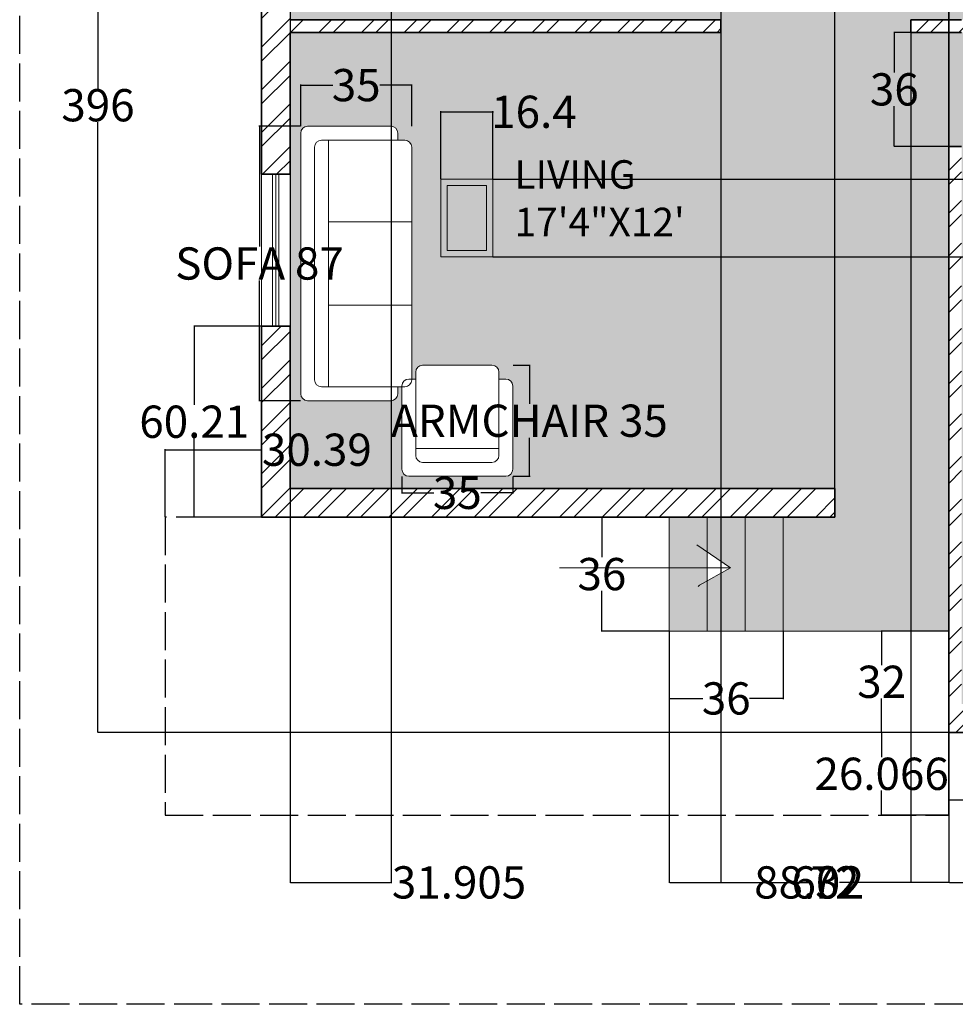
# Model space of a CAD drawing. Units: inches. Extents: x 1410 to 1959, y 5441 to 5968.
# Tile 1 of 5: x 1410 to 1705, y 5441 to 5751. Entities that reach past the tile are written whole.
import ezdxf

# ---------------------------------------------------------------- set-up
doc = ezdxf.new("R2010")
doc.units = ezdxf.units.IN
doc.linetypes.add('ACAD_ISO02W100', pattern=[15, 12, -3])
doc.layers.get('Defpoints').update_dxf_attribs({"linetype": 'ACAD_ISO02W100'})
for name, color, linetype, lineweight in [('00 FURNITURE', 15, 'Continuous', 15), ('A-ANNO-DIMS', 2, 'Continuous', 18), ('A-ANNO-SYMB', 7, 'Continuous', 18), ('A-AREA-IDEN', 7, 'Continuous', 18), ('A-FLOR-STRS', 7, 'Continuous', 18), ('A-WALL', 7, 'Continuous', 35), ('A-WALL-PATT', 8, 'Continuous', 13), ('WINDOW', 160, 'Continuous', 13)]:
    doc.layers.add(name, color=color, linetype=linetype, lineweight=lineweight)
for name, color, linetype, lineweight, true_color in [('A-FLOR-PATT', 9, 'Continuous', 9, 0xafd9aa), ('A-FLOR-STRS-PATT', 254, 'Continuous', 9, 0xddb3d4), ('A-FURN-PATT', 252, 'Continuous', 9, 0x939598)]:
    doc.layers.add(name, color=color, linetype=linetype, lineweight=lineweight, true_color=true_color)
doc.styles.get("Standard").update_dxf_attribs({"font": 'arial.ttf'})
doc.dimstyles.get("Standard").update_dxf_attribs({"dimtxt": 10.18, "dimasz": 0.18, "dimexe": 0.18, "dimexo": 0.0625, "dimgap": 0.09, "dimtad": 0, "dimtih": 1, "dimtoh": 1, "dimdec": 0, "dimzin": 0, "dimdsep": 46, "dimlunit": 3, "dimtxsty": 'Standard', "dimcen": 0.09, "dimadec": 0, "dimazin": 0, "dimtfac": 1, "dimtdec": 0, "dimtofl": 0, "dimtmove": 0, "dimatfit": 3, "dimfxl": 1, "dimtolj": 1, "dimtzin": 0, "dimarcsym": 0})

# ---------------------------------------------------------------- blocks, each defined once
blk = doc.blocks.new('sofa 6')
for p, q in [((-1044.4, 890), (1044.4, 890)), ((-1100, 166.9), (-1100, 834.3)), ((1100, 834.3), (1100, 166.9)), ((-988.8, 55.6), (-988.8, 723.1)), ((-933.1, 778.7), (933.1, 778.7)), ((988.8, 723.1), (988.8, 55.6)), ((-988.8, 667.5), (988.8, 667.5)), ((-333.8, 667.5), (-333.8, 0)), ((333.7, 667.5), (333.7, 0)), ((-988.8, 111.2), (-1044.4, 111.2)), ((1044.4, 111.2), (988.8, 111.2)), ((933.1, 0), (-933.1, 0))]:
    blk.add_line(p, q)
for centre, start, end in [((-1044.4, 834.3), 90, 180), ((1044.4, 834.3), 0, 90), ((-933.1, 723.1), 90, 180), ((933.1, 723.1), 0, 90), ((-1044.4, 166.9), 180, 270), ((1044.4, 166.9), 270, 0), ((-933.1, 55.6), 180, 270), ((933.1, 55.6), 270, 0)]:
    blk.add_arc(centre, 55.6, start, end)
blk = doc.blocks.new('CHAIR')
at = {"layer": '00 FURNITURE'}
for p, q in [((1776.1, 2600.27), (1776.1, 2626.55)), ((1778.29, 2628.74), (1800.19, 2628.74)), ((1802.38, 2626.55), (1802.38, 2600.27)), ((1773.91, 2624.36), (1776.1, 2624.36)), ((1802.38, 2624.36), (1804.57, 2624.36)), ((1771.72, 2595.89), (1771.72, 2622.17)), ((1806.76, 2622.17), (1806.76, 2595.89)), ((1802.38, 2602.46), (1776.1, 2602.46)), ((1800.19, 2598.08), (1778.29, 2598.08)), ((1804.57, 2593.7), (1773.91, 2593.7))]:
    blk.add_line(p, q, dxfattribs=at)
for centre, start, end in [((1778.29, 2626.55), 90, 180), ((1800.19, 2626.55), 0, 90), ((1773.91, 2622.17), 90, 180), ((1804.57, 2622.17), 0, 90), ((1778.29, 2600.27), 180, 270), ((1800.19, 2600.27), 270, 0), ((1773.91, 2595.89), 180, 270), ((1804.57, 2595.89), 270, 0)]:
    blk.add_arc(centre, 2.19, start, end, dxfattribs=at)
blk = doc.blocks.new('WIN-48IN')
for p, q in [((48, 9), (0, 9)), ((0, 5.5), (48, 5.5)), ((0, 4.5), (48, 4.5)), ((0, 3.5), (48, 3.5)), ((0, 0), (48, 0))]:
    blk.add_line(p, q)
blk = doc.blocks.new('*D16')
at = {"layer": 'A-ANNO-DIMS', "color": 0, "lineweight": -2, "transparency": 16777216}
for p, q in [((1498.38, 5717.72), (1485.27, 5717.72)), ((1485.45, 5717.54), (1485.45, 5679.77)), ((1485.45, 5631.29), (1485.45, 5669.06)), ((1498.38, 5631.11), (1485.27, 5631.11))]:
    blk.add_line(p, q, dxfattribs=at)
at = {"layer": 'A-ANNO-DIMS', "color": 0, "transparency": 16777216}
for points in [[(1485.42, 5717.54), (1485.48, 5717.54), (1485.45, 5717.72)], [(1485.42, 5631.29), (1485.48, 5631.29), (1485.45, 5631.11)]]:
    blk.add_solid(points, dxfattribs=at)
at = {"layer": 'Defpoints', "color": 0, "transparency": 16777216}
for p in [(1498.45, 5717.72), (1485.45, 5631.11), (1498.45, 5631.11)]:
    blk.add_point(p, dxfattribs=at)
at = {"layer": 'A-ANNO-DIMS', "color": 0, "transparency": 16777216, "insert": (1485.45, 5674.41), "char_height": 10.18, "attachment_point": 5}
blk.add_mtext('\\A1;SOFA 87', dxfattribs=at)
blk = doc.blocks.new('*D17')
at = {"layer": 'A-ANNO-DIMS', "color": 0, "lineweight": -2, "transparency": 16777216}
for p, q in [((1498.45, 5717.78), (1498.45, 5730.89)), ((1498.63, 5730.71), (1508.55, 5730.71)), ((1533.3, 5730.71), (1523.38, 5730.71)), ((1533.48, 5717.78), (1533.48, 5730.89))]:
    blk.add_line(p, q, dxfattribs=at)
at = {"layer": 'A-ANNO-DIMS', "color": 0, "transparency": 16777216}
for points in [[(1498.63, 5730.74), (1498.63, 5730.68), (1498.45, 5730.71)], [(1533.3, 5730.74), (1533.3, 5730.68), (1533.48, 5730.71)]]:
    blk.add_solid(points, dxfattribs=at)
at = {"layer": 'Defpoints', "color": 0, "transparency": 16777216}
for p in [(1498.45, 5730.71), (1498.45, 5717.72), (1533.48, 5717.72)]:
    blk.add_point(p, dxfattribs=at)
at = {"layer": 'A-ANNO-DIMS', "color": 0, "transparency": 16777216, "insert": (1515.97, 5730.71), "char_height": 10.18, "attachment_point": 5}
blk.add_mtext('\\A1;35', dxfattribs=at)
blk = doc.blocks.new('*D18')
at = {"layer": 'A-ANNO-DIMS', "color": 0, "lineweight": -2, "transparency": 16777216}
for p, q in [((1565.47, 5642.3), (1570.84, 5642.3)), ((1570.66, 5642.12), (1570.66, 5630.14)), ((1570.66, 5607.44), (1570.66, 5619.42)), ((1565.47, 5607.26), (1570.84, 5607.26))]:
    blk.add_line(p, q, dxfattribs=at)
at = {"layer": 'A-ANNO-DIMS', "color": 0, "transparency": 16777216}
for points in [[(1570.63, 5642.12), (1570.69, 5642.12), (1570.66, 5642.3)], [(1570.63, 5607.44), (1570.69, 5607.44), (1570.66, 5607.26)]]:
    blk.add_solid(points, dxfattribs=at)
at = {"layer": 'Defpoints', "color": 0, "transparency": 16777216}
for p in [(1565.4, 5642.3), (1570.66, 5642.3), (1565.4, 5607.26)]:
    blk.add_point(p, dxfattribs=at)
at = {"layer": 'A-ANNO-DIMS', "color": 0, "transparency": 16777216, "insert": (1570.66, 5624.78), "char_height": 10.18, "attachment_point": 5}
blk.add_mtext('\\A1;ARMCHAIR 35', dxfattribs=at)
blk = doc.blocks.new('*D19')
at = {"layer": 'A-ANNO-DIMS', "color": 0, "lineweight": -2, "transparency": 16777216}
for p, q in [((1530.37, 5607.2), (1530.37, 5601.83)), ((1565.4, 5607.2), (1565.4, 5601.83)), ((1530.55, 5602.01), (1540.47, 5602.01)), ((1565.22, 5602.01), (1555.3, 5602.01))]:
    blk.add_line(p, q, dxfattribs=at)
at = {"layer": 'A-ANNO-DIMS', "color": 0, "transparency": 16777216}
for points in [[(1530.55, 5602.04), (1530.55, 5601.98), (1530.37, 5602.01)], [(1565.22, 5602.04), (1565.22, 5601.98), (1565.4, 5602.01)]]:
    blk.add_solid(points, dxfattribs=at)
at = {"layer": 'Defpoints', "color": 0, "transparency": 16777216}
for p in [(1530.37, 5607.26), (1565.4, 5607.26), (1565.4, 5602.01)]:
    blk.add_point(p, dxfattribs=at)
at = {"layer": 'A-ANNO-DIMS', "color": 0, "transparency": 16777216, "insert": (1547.89, 5602.01), "char_height": 10.18, "attachment_point": 5}
blk.add_mtext('\\A1;35', dxfattribs=at)
blk = doc.blocks.new('*D25')
at = {"layer": 'A-ANNO-DIMS', "color": 0, "lineweight": -2, "transparency": 16777216}
for p, q in [((1486.03, 5922.37), (1434.27, 5922.37)), ((1434.45, 5922.19), (1434.45, 5729.66)), ((1434.45, 5526.55), (1434.45, 5719.07)), ((1703.03, 5526.37), (1434.27, 5526.37))]:
    blk.add_line(p, q, dxfattribs=at)
at = {"layer": 'A-ANNO-DIMS', "color": 0, "transparency": 16777216}
for points in [[(1434.42, 5922.19), (1434.48, 5922.19), (1434.45, 5922.37)], [(1434.42, 5526.55), (1434.48, 5526.55), (1434.45, 5526.37)]]:
    blk.add_solid(points, dxfattribs=at)
at = {"layer": 'Defpoints', "color": 0, "transparency": 16777216}
for p in [(1434.45, 5922.37), (1486.09, 5922.37), (1703.09, 5526.37)]:
    blk.add_point(p, dxfattribs=at)
at = {"layer": 'A-ANNO-DIMS', "color": 0, "transparency": 16777216, "insert": (1434.45, 5724.37), "char_height": 10.18, "attachment_point": 5}
blk.add_mtext('\\A1;396', dxfattribs=at)
blk = doc.blocks.new('*D26')
at = {"layer": 'A-ANNO-DIMS', "color": 0, "lineweight": -2, "transparency": 16777216}
for p, q in [((1703.09, 5526.3), (1703.09, 5478.87)), ((1858.09, 5526.3), (1858.09, 5478.87)), ((1703.27, 5479.05), (1769.7, 5479.05)), ((1857.91, 5479.05), (1791.49, 5479.05))]:
    blk.add_line(p, q, dxfattribs=at)
at = {"layer": 'A-ANNO-DIMS', "color": 0, "transparency": 16777216}
for points in [[(1703.27, 5479.08), (1703.27, 5479.02), (1703.09, 5479.05)], [(1857.91, 5479.08), (1857.91, 5479.02), (1858.09, 5479.05)]]:
    blk.add_solid(points, dxfattribs=at)
at = {"layer": 'Defpoints', "color": 0, "transparency": 16777216}
for p in [(1703.09, 5526.37), (1858.09, 5526.37), (1858.09, 5479.05)]:
    blk.add_point(p, dxfattribs=at)
at = {"layer": 'A-ANNO-DIMS', "color": 0, "transparency": 16777216, "insert": (1780.59, 5479.05), "char_height": 10.18, "attachment_point": 5}
blk.add_mtext('\\A1;155', dxfattribs=at)
blk = doc.blocks.new('*D27')
at = {"layer": 'A-ANNO-DIMS', "color": 0, "lineweight": -2, "transparency": 16777216}
for p, q in [((1495.09, 5913.3), (1495.09, 5478.87)), ((1527, 5913.3), (1527, 5478.87)), ((1495.27, 5479.05), (1526.82, 5479.05)), ((1527, 5479.05), (1527.18, 5479.05))]:
    blk.add_line(p, q, dxfattribs=at)
at = {"layer": 'A-ANNO-DIMS', "color": 0, "transparency": 16777216}
for points in [[(1495.27, 5479.08), (1495.27, 5479.02), (1495.09, 5479.05)], [(1526.82, 5479.08), (1526.82, 5479.02), (1527, 5479.05)]]:
    blk.add_solid(points, dxfattribs=at)
at = {"layer": 'Defpoints', "color": 0, "transparency": 16777216}
for p in [(1495.09, 5913.37), (1527, 5913.37), (1527, 5479.05)]:
    blk.add_point(p, dxfattribs=at)
at = {"layer": 'A-ANNO-DIMS', "color": 0, "transparency": 16777216, "insert": (1548.43, 5479.05), "char_height": 10.18, "attachment_point": 5}
blk.add_mtext('\\A1;31.905', dxfattribs=at)
blk = doc.blocks.new('*D30')
at = {"layer": 'A-ANNO-DIMS', "color": 0, "lineweight": -2, "transparency": 16777216}
for p, q in [((1486.04, 5654.58), (1464.67, 5654.58)), ((1464.85, 5654.4), (1464.85, 5629.76)), ((1464.84, 5594.55), (1464.85, 5619.19)), ((1486.03, 5594.37), (1464.66, 5594.37))]:
    blk.add_line(p, q, dxfattribs=at)
at = {"layer": 'A-ANNO-DIMS', "color": 0, "transparency": 16777216}
for points in [[(1464.82, 5654.4), (1464.88, 5654.4), (1464.85, 5654.58)], [(1464.81, 5594.55), (1464.87, 5594.55), (1464.84, 5594.37)]]:
    blk.add_solid(points, dxfattribs=at)
at = {"layer": 'Defpoints', "color": 0, "transparency": 16777216}
for p in [(1464.85, 5654.58), (1486.1, 5654.58), (1486.09, 5594.37)]:
    blk.add_point(p, dxfattribs=at)
at = {"layer": 'A-ANNO-DIMS', "color": 0, "transparency": 16777216, "insert": (1464.85, 5624.47), "char_height": 10.18, "attachment_point": 5}
blk.add_mtext('\\A1;60.21', dxfattribs=at)
blk = doc.blocks.new('*D31')
at = {"layer": 'A-ANNO-DIMS', "color": 0, "lineweight": -2, "transparency": 16777216}
for p, q in [((1703.09, 5526.3), (1703.09, 5504.94)), ((1754.54, 5526.3), (1754.54, 5504.94)), ((1703.27, 5505.12), (1711.51, 5505.12)), ((1754.36, 5505.12), (1746.12, 5505.12))]:
    blk.add_line(p, q, dxfattribs=at)
at = {"layer": 'A-ANNO-DIMS', "color": 0, "transparency": 16777216}
for points in [[(1703.27, 5505.15), (1703.27, 5505.09), (1703.09, 5505.12)], [(1754.36, 5505.15), (1754.36, 5505.09), (1754.54, 5505.12)]]:
    blk.add_solid(points, dxfattribs=at)
at = {"layer": 'Defpoints', "color": 0, "transparency": 16777216}
for p in [(1703.09, 5526.37), (1754.54, 5526.37), (1703.09, 5505.12)]:
    blk.add_point(p, dxfattribs=at)
at = {"layer": 'A-ANNO-DIMS', "color": 0, "transparency": 16777216, "insert": (1728.82, 5505.12), "char_height": 10.18, "attachment_point": 5}
blk.add_mtext('\\A1;51.45', dxfattribs=at)
blk = doc.blocks.new('*D34')
at = {"layer": 'A-ANNO-DIMS', "color": 0, "lineweight": -2, "transparency": 16777216}
for p, q in [((1631.09, 5787.3), (1631.09, 5478.87)), ((1703.09, 5787.3), (1703.09, 5478.87)), ((1631.27, 5479.05), (1659.81, 5479.05)), ((1702.91, 5479.05), (1674.38, 5479.05))]:
    blk.add_line(p, q, dxfattribs=at)
at = {"layer": 'A-ANNO-DIMS', "color": 0, "transparency": 16777216}
for points in [[(1631.27, 5479.08), (1631.27, 5479.02), (1631.09, 5479.05)], [(1702.91, 5479.08), (1702.91, 5479.02), (1703.09, 5479.05)]]:
    blk.add_solid(points, dxfattribs=at)
at = {"layer": 'Defpoints', "color": 0, "transparency": 16777216}
for p in [(1631.09, 5787.37), (1703.09, 5787.37), (1703.09, 5479.05)]:
    blk.add_point(p, dxfattribs=at)
at = {"layer": 'A-ANNO-DIMS', "color": 0, "transparency": 16777216, "insert": (1667.09, 5479.05), "char_height": 10.18, "attachment_point": 5}
blk.add_mtext('\\A1;72', dxfattribs=at)
blk = doc.blocks.new('*D36')
at = {"layer": 'A-ANNO-DIMS', "color": 0, "lineweight": -2, "transparency": 16777216}
for p, q in [((1631.09, 5747.3), (1631.09, 5478.87)), ((1691.09, 5747.3), (1691.09, 5478.87)), ((1631.27, 5479.05), (1653.7, 5479.05)), ((1690.91, 5479.05), (1668.49, 5479.05))]:
    blk.add_line(p, q, dxfattribs=at)
at = {"layer": 'A-ANNO-DIMS', "color": 0, "transparency": 16777216}
for points in [[(1631.27, 5479.08), (1631.27, 5479.02), (1631.09, 5479.05)], [(1690.91, 5479.08), (1690.91, 5479.02), (1691.09, 5479.05)]]:
    blk.add_solid(points, dxfattribs=at)
at = {"layer": 'Defpoints', "color": 0, "transparency": 16777216}
for p in [(1631.09, 5747.37), (1691.09, 5747.37), (1691.09, 5479.05)]:
    blk.add_point(p, dxfattribs=at)
at = {"layer": 'A-ANNO-DIMS', "color": 0, "transparency": 16777216, "insert": (1661.09, 5479.05), "char_height": 10.18, "attachment_point": 5}
blk.add_mtext('\\A1;60', dxfattribs=at)
blk = doc.blocks.new('*D37')
at = {"layer": 'A-ANNO-DIMS', "color": 0, "lineweight": -2, "transparency": 16777216}
for p, q in [((1667.09, 5594.43), (1667.09, 5943.8)), ((1667.27, 5943.62), (1677.72, 5943.62)), ((1702.91, 5943.62), (1692.47, 5943.62)), ((1703.09, 5558.43), (1703.09, 5943.8))]:
    blk.add_line(p, q, dxfattribs=at)
at = {"layer": 'A-ANNO-DIMS', "color": 0, "transparency": 16777216}
for points in [[(1667.27, 5943.65), (1667.27, 5943.59), (1667.09, 5943.62)], [(1702.91, 5943.65), (1702.91, 5943.59), (1703.09, 5943.62)]]:
    blk.add_solid(points, dxfattribs=at)
at = {"layer": 'Defpoints', "color": 0, "transparency": 16777216}
for p in [(1703.09, 5943.62), (1667.09, 5594.37), (1703.09, 5558.37)]:
    blk.add_point(p, dxfattribs=at)
at = {"layer": 'A-ANNO-DIMS', "color": 0, "transparency": 16777216, "insert": (1685.09, 5943.62), "char_height": 10.18, "attachment_point": 5}
blk.add_mtext('\\A1;36', dxfattribs=at)
blk = doc.blocks.new('*D38')
at = {"layer": 'A-ANNO-DIMS', "color": 0, "lineweight": -2, "transparency": 16777216}
for p, q in [((1614.72, 5594.37), (1593.35, 5594.37)), ((1593.53, 5594.19), (1593.53, 5581.66)), ((1593.53, 5558.55), (1593.53, 5571.07)), ((1614.72, 5558.37), (1593.35, 5558.37))]:
    blk.add_line(p, q, dxfattribs=at)
at = {"layer": 'A-ANNO-DIMS', "color": 0, "transparency": 16777216}
for points in [[(1593.5, 5594.19), (1593.56, 5594.19), (1593.53, 5594.37)], [(1593.5, 5558.55), (1593.56, 5558.55), (1593.53, 5558.37)]]:
    blk.add_solid(points, dxfattribs=at)
at = {"layer": 'Defpoints', "color": 0, "transparency": 16777216}
for p in [(1593.53, 5594.37), (1614.78, 5594.37), (1614.78, 5558.37)]:
    blk.add_point(p, dxfattribs=at)
at = {"layer": 'A-ANNO-DIMS', "color": 0, "transparency": 16777216, "insert": (1593.53, 5576.37), "char_height": 10.18, "attachment_point": 5}
blk.add_mtext('\\A1;36', dxfattribs=at)
blk = doc.blocks.new('*D39')
at = {"layer": 'A-ANNO-DIMS', "color": 0, "lineweight": -2, "transparency": 16777216}
for p, q in [((1614.78, 5558.3), (1614.78, 5478.87)), ((1703.09, 5558.3), (1703.09, 5478.87)), ((1614.96, 5479.05), (1641.72, 5479.05)), ((1702.91, 5479.05), (1676.16, 5479.05))]:
    blk.add_line(p, q, dxfattribs=at)
at = {"layer": 'A-ANNO-DIMS', "color": 0, "transparency": 16777216}
for points in [[(1614.96, 5479.08), (1614.96, 5479.02), (1614.78, 5479.05)], [(1702.91, 5479.08), (1702.91, 5479.02), (1703.09, 5479.05)]]:
    blk.add_solid(points, dxfattribs=at)
at = {"layer": 'Defpoints', "color": 0, "transparency": 16777216}
for p in [(1614.78, 5558.37), (1703.09, 5558.37), (1703.09, 5479.05)]:
    blk.add_point(p, dxfattribs=at)
at = {"layer": 'A-ANNO-DIMS', "color": 0, "transparency": 16777216, "insert": (1658.94, 5479.05), "char_height": 10.18, "attachment_point": 5}
blk.add_mtext('\\A1;88.32', dxfattribs=at)
blk = doc.blocks.new('*D40')
at = {"layer": 'A-ANNO-DIMS', "color": 0, "lineweight": -2, "transparency": 16777216}
for p, q in [((1703.03, 5558.37), (1681.66, 5558.37)), ((1681.84, 5558.19), (1681.84, 5547.66)), ((1681.84, 5526.55), (1681.84, 5537.07)), ((1703.03, 5526.37), (1681.66, 5526.37))]:
    blk.add_line(p, q, dxfattribs=at)
at = {"layer": 'A-ANNO-DIMS', "color": 0, "transparency": 16777216}
for points in [[(1681.81, 5558.19), (1681.87, 5558.19), (1681.84, 5558.37)], [(1681.81, 5526.55), (1681.87, 5526.55), (1681.84, 5526.37)]]:
    blk.add_solid(points, dxfattribs=at)
at = {"layer": 'Defpoints', "color": 0, "transparency": 16777216}
for p in [(1681.84, 5558.37), (1703.09, 5558.37), (1703.09, 5526.37)]:
    blk.add_point(p, dxfattribs=at)
at = {"layer": 'A-ANNO-DIMS', "color": 0, "transparency": 16777216, "insert": (1681.84, 5542.37), "char_height": 10.18, "attachment_point": 5}
blk.add_mtext('\\A1;32', dxfattribs=at)
blk = doc.blocks.new('*D47')
at = {"layer": 'A-ANNO-DIMS', "color": 0, "lineweight": -2, "transparency": 16777216}
for p, q in [((1707.03, 5747.37), (1685.66, 5747.37)), ((1685.84, 5747.19), (1685.84, 5734.66)), ((1685.84, 5711.55), (1685.84, 5724.07)), ((1707.03, 5711.37), (1685.66, 5711.37))]:
    blk.add_line(p, q, dxfattribs=at)
at = {"layer": 'A-ANNO-DIMS', "color": 0, "transparency": 16777216}
for points in [[(1685.81, 5747.19), (1685.87, 5747.19), (1685.84, 5747.37)], [(1685.81, 5711.55), (1685.87, 5711.55), (1685.84, 5711.37)]]:
    blk.add_solid(points, dxfattribs=at)
at = {"layer": 'Defpoints', "color": 0, "transparency": 16777216}
for p in [(1685.84, 5747.37), (1707.09, 5747.37), (1707.09, 5711.37)]:
    blk.add_point(p, dxfattribs=at)
at = {"layer": 'A-ANNO-DIMS', "color": 0, "transparency": 16777216, "insert": (1685.84, 5729.37), "char_height": 10.18, "attachment_point": 5}
blk.add_mtext('\\A1;36', dxfattribs=at)
blk = doc.blocks.new('*D53')
at = {"layer": 'A-ANNO-DIMS', "color": 0, "lineweight": -2, "transparency": 16777216}
for p, q in [((1455.7, 5594.43), (1455.7, 5615.8)), ((1455.88, 5615.62), (1485.92, 5615.62)), ((1486.09, 5594.43), (1486.1, 5615.8)), ((1486.1, 5615.62), (1486.28, 5615.62))]:
    blk.add_line(p, q, dxfattribs=at)
at = {"layer": 'A-ANNO-DIMS', "color": 0, "transparency": 16777216}
for points in [[(1455.88, 5615.65), (1455.88, 5615.59), (1455.7, 5615.62)], [(1485.92, 5615.65), (1485.92, 5615.59), (1486.1, 5615.62)]]:
    blk.add_solid(points, dxfattribs=at)
at = {"layer": 'Defpoints', "color": 0, "transparency": 16777216}
for p in [(1486.1, 5615.62), (1455.7, 5594.37), (1486.09, 5594.37)]:
    blk.add_point(p, dxfattribs=at)
at = {"layer": 'A-ANNO-DIMS', "color": 0, "transparency": 16777216, "insert": (1503.55, 5615.62), "char_height": 10.18, "attachment_point": 5}
blk.add_mtext('\\A1;30.39', dxfattribs=at)
blk = doc.blocks.new('*D54')
at = {"layer": 'A-ANNO-DIMS', "color": 0, "lineweight": -2, "transparency": 16777216}
for p, q in [((1703.03, 5526.37), (1681.66, 5526.37)), ((1681.84, 5526.19), (1681.84, 5518.62)), ((1681.84, 5500.48), (1681.84, 5508.05)), ((1703.03, 5500.3), (1681.66, 5500.3))]:
    blk.add_line(p, q, dxfattribs=at)
at = {"layer": 'A-ANNO-DIMS', "color": 0, "transparency": 16777216}
for points in [[(1681.81, 5526.19), (1681.87, 5526.19), (1681.84, 5526.37)], [(1681.81, 5500.48), (1681.87, 5500.48), (1681.84, 5500.3)]]:
    blk.add_solid(points, dxfattribs=at)
at = {"layer": 'Defpoints', "color": 0, "transparency": 16777216}
for p in [(1681.84, 5526.37), (1703.09, 5526.37), (1703.09, 5500.3)]:
    blk.add_point(p, dxfattribs=at)
at = {"layer": 'A-ANNO-DIMS', "color": 0, "transparency": 16777216, "insert": (1681.84, 5513.33), "char_height": 10.18, "attachment_point": 5}
blk.add_mtext('\\A1;26.066', dxfattribs=at)
blk = doc.blocks.new('*D55')
at = {"layer": 'A-ANNO-DIMS', "color": 0, "lineweight": -2, "transparency": 16777216}
for p, q in [((1614.78, 5558.3), (1614.78, 5536.94)), ((1650.78, 5558.3), (1650.78, 5536.94)), ((1614.96, 5537.12), (1625.4, 5537.12)), ((1650.6, 5537.12), (1640.15, 5537.12))]:
    blk.add_line(p, q, dxfattribs=at)
at = {"layer": 'A-ANNO-DIMS', "color": 0, "transparency": 16777216}
for points in [[(1614.96, 5537.15), (1614.96, 5537.09), (1614.78, 5537.12)], [(1650.6, 5537.15), (1650.6, 5537.09), (1650.78, 5537.12)]]:
    blk.add_solid(points, dxfattribs=at)
at = {"layer": 'Defpoints', "color": 0, "transparency": 16777216}
for p in [(1614.78, 5558.37), (1650.78, 5558.37), (1614.78, 5537.12)]:
    blk.add_point(p, dxfattribs=at)
at = {"layer": 'A-ANNO-DIMS', "color": 0, "transparency": 16777216, "insert": (1632.78, 5537.12), "char_height": 10.18, "attachment_point": 5}
blk.add_mtext('\\A1;36', dxfattribs=at)
blk = doc.blocks.new('*D59')
at = {"layer": 'A-ANNO-DIMS', "color": 0, "lineweight": -2, "transparency": 16777216}
for p, q in [((1559.15, 5701.04), (1879.55, 5701.04)), ((1879.37, 5700.86), (1879.37, 5694.04)), ((1879.37, 5676.64), (1879.37, 5683.46)), ((1559.15, 5676.46), (1879.55, 5676.46))]:
    blk.add_line(p, q, dxfattribs=at)
at = {"layer": 'A-ANNO-DIMS', "color": 0, "transparency": 16777216}
for points in [[(1879.34, 5700.86), (1879.4, 5700.86), (1879.37, 5701.04)], [(1879.34, 5676.64), (1879.4, 5676.64), (1879.37, 5676.46)]]:
    blk.add_solid(points, dxfattribs=at)
at = {"layer": 'Defpoints', "color": 0, "transparency": 16777216}
for p in [(1559.09, 5701.04), (1559.09, 5676.46), (1879.37, 5676.46)]:
    blk.add_point(p, dxfattribs=at)
at = {"layer": 'A-ANNO-DIMS', "color": 0, "transparency": 16777216, "insert": (1879.37, 5688.75), "char_height": 10.18, "attachment_point": 5}
blk.add_mtext('\\A1;24.58', dxfattribs=at)
blk = doc.blocks.new('*D60')
at = {"layer": 'A-ANNO-DIMS', "color": 0, "lineweight": -2, "transparency": 16777216}
for p, q in [((1542.69, 5701.1), (1542.69, 5722.47)), ((1542.87, 5722.29), (1558.91, 5722.29)), ((1559.09, 5701.1), (1559.09, 5722.47)), ((1559.09, 5722.29), (1559.27, 5722.29))]:
    blk.add_line(p, q, dxfattribs=at)
at = {"layer": 'A-ANNO-DIMS', "color": 0, "transparency": 16777216}
for points in [[(1542.87, 5722.32), (1542.87, 5722.26), (1542.69, 5722.29)], [(1558.91, 5722.32), (1558.91, 5722.26), (1559.09, 5722.29)]]:
    blk.add_solid(points, dxfattribs=at)
at = {"layer": 'Defpoints', "color": 0, "transparency": 16777216}
for p in [(1559.09, 5722.29), (1542.69, 5701.04), (1559.09, 5701.04)]:
    blk.add_point(p, dxfattribs=at)
at = {"layer": 'A-ANNO-DIMS', "color": 0, "transparency": 16777216, "insert": (1572.08, 5722.29), "char_height": 10.18, "attachment_point": 5}
blk.add_mtext('\\A1;16.4', dxfattribs=at)

msp = doc.modelspace()

# ---------------------------------------------------------------- hatches: boundary and pattern name
at = {"layer": 'A-FLOR-PATT', "transparency": 33554534}
h = msp.add_hatch(color=256, dxfattribs=at)
h.dxf.hatch_style = 1
h.paths.add_polyline_path([(1849.0942, 5913.3659), (1817.1029, 5913.3659), (1769.1029, 5913.3659), (1769.1029, 5913.3659), (1707.0942, 5913.3659), (1707.0942, 5787.3659), (1703.0942, 5787.3659), (1703.0942, 5799.3659), (1631.0942, 5799.3659), (1631.0942, 5787.3659), (1627.0942, 5787.3659), (1627.0942, 5889.3659), (1519.0989, 5889.3659), (1519.0989, 5816.4745), (1495.0981, 5816.4745), (1495.0981, 5809.856), (1495.0942, 5751.3659), (1631.0942, 5751.3659), (1631.0942, 5747.3659), (1495.0942, 5747.3659), (1495.0942, 5702.5811), (1495.0984, 5654.5768), (1495.0942, 5603.3659), (1667.0942, 5603.3659), (1667.0942, 5594.3659), (1650.778, 5594.3659), (1650.778, 5558.3659), (1703.0942, 5558.3659), (1703.0942, 5594.3659), (1703.0942, 5711.3659), (1707.0942, 5711.3659), (1707.0942, 5535.3659), (1754.5413, 5535.3659), (1802.541, 5535.3658), (1802.5413, 5535.3658), (1802.5413, 5535.3659), (1849.0942, 5535.3659), (1849.0942, 5651.3659), (1743.0942, 5651.3659), (1743.0942, 5655.3659), (1849.0942, 5655.3659), (1849.0942, 5665.4579), (1849.0942, 5689.4579), (1849.0942, 5699.3659), (1801.0942, 5699.3659), (1801.0942, 5685.3659), (1797.0942, 5685.3659), (1797.0942, 5699.3659), (1783.0942, 5699.3659), (1783.0942, 5703.3659), (1849.0942, 5703.3659), (1849.0942, 5716.9764), (1849.123, 5716.9764), (1849.123, 5740.9654), (1849.0942, 5740.9654), (1849.0942, 5747.3659), (1753.0942, 5747.3659), (1753.0942, 5699.3659), (1749.0942, 5699.3659), (1749.0942, 5747.3659), (1707.0942, 5747.3659), (1691.0942, 5747.3659), (1691.0942, 5751.3659), (1707.0942, 5751.3659), (1849.0942, 5751.3659)])
h.paths.add_polyline_path([(1533.4842, 5711.1518), (1533.4842, 5637.9201), (1534.7464, 5637.9201), (1534.7464, 5640.1099, -0.41421356), (1536.9363, 5642.2998), (1558.8347, 5642.2998, -0.41421356), (1561.0246, 5640.1099), (1561.0246, 5637.9201), (1563.2144, 5637.9201, -0.41421356), (1565.4042, 5635.7302), (1565.4042, 5609.4519, -0.41421356), (1563.2144, 5607.2621), (1532.5566, 5607.2621, -0.41421356), (1530.3668, 5609.4519), (1530.3668, 5635.4862), (1529.1045, 5635.4862), (1529.1045, 5633.2964, -0.41421356), (1526.9147, 5631.1065), (1500.6363, 5631.1065, -0.41421356), (1498.4465, 5633.2964), (1498.4465, 5715.5315, -0.41421356), (1500.6363, 5717.7213), (1526.9147, 5717.7213, -0.41421356), (1529.1045, 5715.5315), (1529.1045, 5713.3417), (1531.2944, 5713.3417, -0.41421356)], flags=16)
h.paths.add_polyline_path([(1771.0631, 5793.9619), (1771.0631, 5835.0118), (1771.0631, 5856.9619, -0.41421356), (1771.9631, 5857.8619), (1842.1181, 5857.8619, -0.41421356), (1843.0181, 5856.9619), (1843.0181, 5857.8619), (1846.6631, 5857.8619), (1846.6631, 5793.0619), (1843.0181, 5793.0619), (1828.4381, 5793.0619), (1771.9631, 5793.0619, -0.41421356)], flags=16)
h.paths.add_polyline_path([(1771.0631, 5805.9671, 0.25346465), (1781.0166, 5803.0153, 0.25379956), (1783.9781, 5793.0522)], flags=16)
h.paths.add_polyline_path([(1746.3058, 5612.0795), (1768.2559, 5612.0795), (1809.3058, 5612.0795, -0.41421356), (1810.2058, 5611.1795), (1810.2058, 5554.7045), (1810.2058, 5540.1245), (1810.2058, 5536.4795), (1745.4058, 5536.4795), (1745.4058, 5540.1245), (1746.3058, 5540.1245, -0.41421356), (1745.4058, 5541.0245), (1745.4058, 5611.1795, -0.41421356)], flags=16)
h.paths.add_polyline_path([(1819.5646, 5793.1537), (1819.5646, 5793.8054, 0.05271893), (1808.0815, 5849.0458, 0.29223153), (1819.5646, 5857.6981), (1828.4381, 5857.6981), (1828.4381, 5857.0464), (1828.4381, 5847.601, -0.06332793), (1838.1593, 5837.9401, -0.38046479), (1838.3062, 5835.5217, -0.02593615), (1834.5989, 5831.2824, -0.02509022), (1838.1593, 5827.1584, -0.38046478), (1838.3062, 5824.74, -0.05941785), (1829.2061, 5815.646, -0.11763956), (1828.4381, 5815.2914), (1828.4381, 5793.1537)], flags=0)
h.paths.add_polyline_path([(1819.5646, 5793.1537), (1819.5646, 5822.5662, -0.01603557), (1817.3363, 5825.2436, -0.4295765), (1817.4052, 5827.8865, -0.01537126), (1819.5646, 5830.4335), (1819.5646, 5833.3479, -0.01603557), (1817.3363, 5836.0254, -0.48413611), (1817.6682, 5838.8652, 0.00079305), (1817.0318, 5838.199, 0.26524804), (1817.0526, 5836.3926, 0.02736634), (1820.9176, 5831.8795, 0.02734261), (1817.0221, 5827.3996, 0.26229506), (1817.0526, 5825.6108, 0.06555279), (1827.0712, 5815.5721), (1827.0712, 5793.1537)], flags=0)
h.paths.add_polyline_path([(1830.4631, 5775.9619), (1830.4631, 5792.1619), (1846.6631, 5792.1619), (1846.6631, 5775.9619)], flags=16)
h.paths.add_polyline_path([(1831.3631, 5776.8619), (1831.3631, 5791.2619), (1845.7631, 5791.2619), (1845.7631, 5776.8619)], flags=0)
h.paths.add_polyline_path([(1836.6983, 5784.1006, -1), (1843.9547, 5784.1006, -1)], flags=0)
h.paths.add_polyline_path([(1819.2615, 5682.5311, -0.25820517), (1830.2865, 5687.0962, -0.1716359), (1835.799, 5683.9093), (1838.1615, 5683.9093), (1838.1615, 5688.0436, -0.41421356), (1839.1458, 5689.028), (1845.4458, 5689.028, -0.41421356), (1846.4302, 5688.0436), (1846.4302, 5671.8999, -0.41421356), (1845.4458, 5670.9155), (1839.1458, 5670.9155, -0.41421356), (1838.1615, 5671.8999), (1838.1615, 5676.0343), (1835.799, 5676.0343, -0.1716359), (1830.2865, 5672.8474, -0.25820517), (1819.2615, 5677.4124)], flags=16)
h.paths.add_polyline_path([(1820.8043, 5682.5681, -0.21038447), (1830.2865, 5685.5212, -0.1716359), (1835.799, 5682.3343), (1835.799, 5677.6093, -0.1716359), (1830.2865, 5674.4224, -0.21038447), (1820.8043, 5677.3755)], flags=0)
h.paths.add_polyline_path([(1842.0614, 5784.0231), (1841.8811, 5784.0231, -0.54460611), (1839.6163, 5782.7155), (1839.5262, 5782.5594, 0.54796211)], flags=0)
h.paths.add_polyline_path([(1840.3713, 5784.1781), (1840.3265, 5784.2556), (1840.2818, 5784.1781)], flags=0)
h.paths.add_polyline_path([(1830.4631, 5858.7619), (1830.4631, 5874.9619), (1846.6631, 5874.9619), (1846.6631, 5858.7619)], flags=16)
h.paths.add_polyline_path([(1831.3631, 5859.6619), (1831.3631, 5874.0619), (1845.7631, 5874.0619), (1845.7631, 5859.6619)], flags=0)
h.paths.add_polyline_path([(1755.6206, 5556.6903, -0.00089292), (1756.3396, 5557.4382), (1745.5695, 5557.4382), (1745.5695, 5554.7045), (1746.2212, 5554.7045), (1755.5673, 5554.7045, -0.38881883)], flags=0)
h.paths.add_polyline_path([(1810.114, 5563.578), (1810.114, 5554.7045), (1809.4622, 5554.7045), (1787.9762, 5554.7045, -0.11778508), (1787.6251, 5553.9338, -0.05941785), (1778.5249, 5544.8398, -0.37985907), (1776.1092, 5544.9833, -0.02509022), (1771.9852, 5548.5437, 0.03343123), (1776.8399, 5553.9365, 0.30845915), (1776.98, 5555.985, 0.04782679), (1769.9197, 5563.578), (1772.8341, 5563.578, -0.01537126), (1775.3811, 5565.7373, -0.4295765), (1778.024, 5565.8063, -0.01603557), (1780.7015, 5563.578)], flags=0)
h.paths.add_polyline_path([(1728.3058, 5552.6795), (1744.5058, 5552.6795), (1744.5058, 5536.4795), (1728.3058, 5536.4795)], flags=16)
h.paths.add_polyline_path([(1810.2058, 5599.1742, 0.25346465), (1800.2523, 5602.126, 0.25379956), (1797.2908, 5612.0892)], flags=16)
h.paths.add_polyline_path([(1843.9547, 5866.8231, -1), (1836.6983, 5866.8231, -1)], flags=0)
h.paths.add_polyline_path([(1729.2058, 5551.7795), (1743.6058, 5551.7795), (1743.6058, 5537.3795), (1729.2058, 5537.3795)], flags=0)
h.paths.add_polyline_path([(1839.4821, 5865.5155), (1840.237, 5866.8231), (1839.4821, 5868.1307, 0.25464572), (1838.77, 5866.8231, 0.25464572)], flags=0)
h.paths.add_polyline_path([(1842.0614, 5866.7456), (1840.3713, 5866.7456), (1839.5262, 5865.2819, 0.54796211)], flags=0)
h.paths.add_polyline_path([(1732.8163, 5542.8161, -1), (1740.0727, 5542.8161, -1)], flags=0)
h.paths.add_polyline_path([(1737.8296, 5543.5262), (1736.522, 5542.7713), (1736.522, 5541.2615, 0.39969799), (1738.001, 5542.8161, 0.11900365)], flags=0)
h.paths.add_polyline_path([(1738.1811, 5542.8161, -1), (1734.7079, 5542.8161, -1)], flags=0)
h.paths.add_polyline_path([(1736.4445, 5542.9056), (1736.367, 5542.9503), (1736.367, 5542.8608)], flags=0)
h.paths.add_polyline_path([(1811.1058, 5552.6795), (1827.3058, 5552.6795), (1827.3058, 5536.4795), (1811.1058, 5536.4795)], flags=16)
h.paths.add_polyline_path([(1812.0058, 5551.7795), (1826.4058, 5551.7795), (1826.4058, 5537.3795), (1812.0058, 5537.3795)], flags=0)
h.paths.add_polyline_path([(1815.5388, 5542.8161, -1), (1822.7952, 5542.8161, -1)], flags=0)
h.paths.add_polyline_path([(1820.5521, 5543.5262), (1819.2445, 5542.7713), (1819.2445, 5541.2615, 0.39969799), (1820.7235, 5542.8161, 0.11900365)], flags=0)
h.paths.add_polyline_path([(1820.9036, 5542.8161, -1), (1817.4304, 5542.8161, -1)], flags=0)
h.paths.add_polyline_path([(1819.167, 5542.9056), (1819.0895, 5542.9503), (1819.0895, 5542.8608)], flags=0)
h.paths.add_polyline_path([(1707.0264, 5710.8395), (1750.0905, 5710.8395), (1750.0905, 5723.2037), (1707.0264, 5723.2037)], flags=25)
h.paths.add_polyline_path([(1786.4108, 5658.162), (1818.7518, 5658.162), (1818.7518, 5680.5262), (1786.4108, 5680.5262)], flags=24)
h.paths.add_polyline_path([(1787.0609, 5715.7465), (1838.4906, 5715.7465), (1838.4906, 5738.1353), (1787.0609, 5738.1353)], flags=24)
h.paths.add_polyline_path([(1743.8116, 5616.0244), (1813.7243, 5616.0244), (1813.7243, 5649.6076), (1743.8116, 5649.6076)], flags=24)
h.paths.add_polyline_path([(1719.2569, 5867.7974), (1789.1696, 5867.7974), (1789.1696, 5901.3806), (1719.2569, 5901.3806)], flags=24)
h.paths.add_polyline_path([(1562.3198, 5677.907), (1619.4324, 5677.907), (1619.4324, 5711.4902), (1562.3198, 5711.4902)], flags=24)
h.paths.add_polyline_path([(1544.1706, 5816.5955), (1604.3036, 5816.5955), (1604.3036, 5850.1787), (1544.1706, 5850.1787)], flags=24)
at = {"layer": 'A-FLOR-STRS-PATT'}
h = msp.add_hatch(color=256, dxfattribs=at)
h.dxf.hatch_style = 1
h.paths.add_polyline_path([(1650.778, 5594.3659), (1638.778, 5594.3659), (1638.778, 5558.3659), (1650.778, 5558.3659)])
h.paths.add_polyline_path([(1638.778, 5594.3659), (1626.778, 5594.3659), (1626.778, 5583.3738), (1634.1392, 5578.3256), (1626.778, 5574.2563), (1626.778, 5558.3659), (1638.778, 5558.3659)])
h.paths.add_polyline_path([(1626.778, 5574.2563), (1626.778, 5578.3256), (1614.778, 5578.3256), (1614.778, 5558.3659), (1626.778, 5558.3659)])
h.paths.add_polyline_path([(1626.778, 5594.3659), (1614.778, 5594.3659), (1614.778, 5578.3256), (1626.778, 5578.3256)])
at = {"layer": 'A-FURN-PATT'}
h = msp.add_hatch(color=256, dxfattribs=at)
h.dxf.hatch_style = 1
h.paths.add_polyline_path([(1559.091, 5701.0417), (1542.6924, 5701.0417), (1542.6924, 5676.4614), (1559.091, 5676.4614)])
h.paths.add_polyline_path([(1557.091, 5699.0417), (1557.091, 5678.4614), (1544.6924, 5678.4614), (1544.6924, 5699.0417)], flags=16)
h = msp.add_hatch(color=256, dxfattribs=at)
h.dxf.hatch_style = 1
h.paths.add_polyline_path([(1557.091, 5699.0417), (1544.6924, 5699.0417), (1544.6924, 5678.4614), (1557.091, 5678.4614)])
at = {"layer": 'A-WALL-PATT'}
h = msp.add_hatch(dxfattribs=at)
h.set_pattern_fill('ANSI32', color=256)
h.paths.add_polyline_path([(1526.9987, 5922.3659), (1486.0942, 5922.3659), (1486.0942, 5857.8561), (1495.0942, 5857.8561), (1495.0942, 5913.3659), (1526.9987, 5913.3659)])
h.paths.add_polyline_path([(1769.1029, 5922.3659), (1574.9987, 5922.3659), (1574.9987, 5913.3659), (1574.9993, 5913.3659), (1627.0942, 5913.3659), (1627.0942, 5787.3659), (1631.0942, 5787.3659), (1631.0942, 5913.3659), (1703.0942, 5913.3659), (1703.0942, 5787.3659), (1707.0942, 5787.3659), (1707.0942, 5913.3659), (1769.1029, 5913.3659)])
h.paths.add_polyline_path([(1858.0942, 5922.3659), (1817.1029, 5922.3659), (1817.1029, 5913.3659), (1849.0942, 5913.3659), (1849.0942, 5751.3659), (1707.0942, 5751.3659), (1691.0942, 5751.3659), (1691.0942, 5747.3659), (1707.0942, 5747.3659), (1849.0942, 5747.3659), (1849.0942, 5740.9764), (1858.0942, 5740.9764)])
h.paths.add_polyline_path([(1495.0942, 5809.8561), (1486.0981, 5809.8561), (1486.0981, 5809.856), (1486.0942, 5702.5811), (1495.0942, 5702.5811), (1495.0942, 5747.3659), (1631.0942, 5747.3659), (1631.0942, 5751.3659), (1495.0942, 5751.3659)])
h.paths.add_polyline_path([(1495.0942, 5654.5811), (1486.0984, 5654.5811), (1486.0984, 5654.5768), (1486.0942, 5594.3659), (1667.0942, 5594.3659), (1667.0942, 5603.3659), (1495.0942, 5603.3659)])
h.paths.add_polyline_path([(1858.0942, 5665.4579), (1849.0942, 5665.4579), (1849.0942, 5655.3659), (1743.0942, 5655.3659), (1743.0942, 5651.3659), (1849.0942, 5651.3659), (1849.0942, 5535.3659), (1802.5413, 5535.3659), (1802.5413, 5526.3659), (1858.0942, 5526.3659)])
h.paths.add_polyline_path([(1858.0942, 5716.9654), (1849.0942, 5716.9654), (1849.0942, 5703.3659), (1783.0942, 5703.3659), (1783.0942, 5699.3659), (1797.0942, 5699.3659), (1797.0942, 5685.3659), (1801.0942, 5685.3659), (1801.0942, 5699.3659), (1849.0942, 5699.3659), (1849.0942, 5689.4579), (1858.0942, 5689.4579)])
h.paths.add_polyline_path([(1753.0942, 5747.3659), (1749.0942, 5747.3659), (1749.0942, 5699.3659), (1753.0942, 5699.3659)])
h.paths.add_polyline_path([(1707.0942, 5711.3659), (1703.0942, 5711.3659), (1703.0942, 5594.3659), (1703.0942, 5526.3659), (1754.5413, 5526.3659), (1754.5413, 5535.3658), (1754.541, 5535.3658), (1707.0942, 5535.3659)])

# ---------------------------------------------------------------- linework, layer by layer
at = {"layer": '00 FURNITURE'}
for points in [[(1542.6924, 5701.0417), (1559.091, 5701.0417), (1559.091, 5676.4614), (1542.6924, 5676.4614)], [(1544.6924, 5699.0417), (1557.091, 5699.0417), (1557.091, 5678.4614), (1544.6924, 5678.4614)]]:
    msp.add_lwpolyline(points, close=True, dxfattribs=at)
at = {"layer": 'A-ANNO-SYMB'}
for p, q in [((1634.1392, 5578.3256), (1623.5064, 5585.6174)), ((1623.5064, 5585.6174), (1634.1392, 5578.3256)), ((1580.1411, 5578.3256), (1634.1392, 5578.3256)), ((1634.1392, 5578.3256), (1624.3403, 5572.9088)), ((1624.3403, 5572.9088), (1623.9234, 5572.4921))]:
    msp.add_line(p, q, dxfattribs=at)
at = {"layer": 'A-FLOR-STRS'}
for p, q in [((1614.778, 5558.3659), (1614.778, 5594.3659)), ((1626.778, 5558.3659), (1626.778, 5594.3659)), ((1638.778, 5558.3659), (1638.778, 5594.3659)), ((1650.778, 5558.3659), (1650.778, 5594.3659)), ((1614.778, 5558.3659), (1703.0942, 5558.3659))]:
    msp.add_line(p, q, dxfattribs=at)
at = {"layer": 'A-WALL'}
for p, q in [((1486.0942, 5702.5811), (1486.0942, 5809.8561)), ((1495.0942, 5751.3659), (1631.0942, 5751.3659)), ((1631.0942, 5747.3659), (1631.0942, 5751.3659)), ((1691.0942, 5751.3659), (1707.0942, 5751.3659)), ((1691.0942, 5747.3659), (1691.0942, 5751.3659)), ((1495.0942, 5747.3659), (1631.0942, 5747.3659)), ((1495.0942, 5702.5811), (1495.0942, 5747.3659)), ((1691.0942, 5747.3659), (1707.0942, 5747.3659)), ((1703.0942, 5711.3659), (1703.0942, 5594.3659)), ((1703.0942, 5711.3659), (1707.0942, 5711.3659)), ((1486.0942, 5702.5811), (1495.0942, 5702.5811)), ((1486.0942, 5594.3659), (1486.0942, 5654.5811)), ((1486.0942, 5654.5811), (1495.0942, 5654.5811)), ((1495.0942, 5603.3659), (1495.0942, 5654.5811)), ((1495.0942, 5603.3659), (1667.0942, 5603.3659)), ((1667.0942, 5603.3659), (1667.0942, 5594.3659)), ((1486.0942, 5594.3659), (1667.0942, 5594.3659)), ((1703.0942, 5594.3659), (1703.0942, 5500.2998)), ((1754.5413, 5526.3659), (1703.0942, 5526.3659))]:
    msp.add_line(p, q, dxfattribs=at)
at = {"layer": 'Defpoints'}
for p, q in [((1486.0928, 5594.3682), (1455.703, 5594.3682)), ((1455.703, 5594.3682), (1455.703, 5500.2998)), ((1455.703, 5500.2998), (1703.0942, 5500.2998))]:
    msp.add_line(p, q, dxfattribs=at)
msp.add_lwpolyline([(1409.7428, 5967.6887), (1920.4745, 5967.6887), (1920.4745, 5440.571), (1409.7428, 5440.571)], close=True, dxfattribs=at)

# ---------------------------------------------------------------- block references
at = {"layer": '00 FURNITURE', "xscale": -0.0393700787401575, "yscale": 0.0393700787401575, "zscale": 0.0393700787401575, "rotation": 90}
msp.add_blockref('sofa 6', (1533.4842, 5674.4139), dxfattribs=at)
at = {"layer": '00 FURNITURE'}
msp.add_blockref('CHAIR', (-241.3535, 3013.5608), dxfattribs=at)
at = {"layer": 'WINDOW', "rotation": 269.9999999999966}
msp.add_blockref('WIN-48IN', (1486.0984, 5702.5768), dxfattribs=at)

# ---------------------------------------------------------------- texts
at = {"layer": 'A-AREA-IDEN', "insert": (1565.9388, 5707.0117), "char_height": 9, "attachment_point": 1}
msp.add_mtext_dynamic_manual_height_columns('LIVING\\P17\'4"X12\'', width=124.909089, gutter_width=12.5, heights=[0], dxfattribs=at)

# ---------------------------------------------------------------- dimensions: what is measured, and where the dimension line sits
at = {"layer": 'A-ANNO-DIMS'}
for base, p1, p2, override, picture, middle in [((1703.0942, 5943.6159), (1667.0942, 5594.3659), (1703.0942, 5558.3659), {"dimdec": 0, "dimlfac": 1, "dimrnd": 0, "dimzin": 0, "dimdsep": 46, "dimlunit": 2}, '*D37', (1685.0942, 5943.6159)), ((1526.9993, 5479.0498), (1495.0942, 5913.3659), (1526.9993, 5913.3659), {"dimdec": 3, "dimlfac": 1, "dimrnd": 0, "dimzin": 0, "dimdsep": 46, "dimlunit": 2}, '*D27', (1548.4348, 5479.0498)), ((1703.0942, 5479.0498), (1631.0942, 5787.3659), (1703.0942, 5787.3659), {"dimdec": 0, "dimlfac": 1, "dimrnd": 0, "dimzin": 0, "dimdsep": 46, "dimlunit": 2}, '*D34', (1667.0942, 5479.0498)), ((1691.0942, 5479.0498), (1631.0942, 5747.3659), (1691.0942, 5747.3659), {"dimdec": 0, "dimlfac": 1, "dimrnd": 0, "dimzin": 0, "dimdsep": 46, "dimlunit": 2}, '*D36', (1661.0942, 5479.0498)), ((1559.091, 5722.2917), (1542.6924, 5701.0417), (1559.091, 5701.0417), {"dimdec": 1, "dimlfac": 1, "dimrnd": 0, "dimzin": 0, "dimdsep": 46, "dimlunit": 2}, '*D60', (1572.0825, 5722.2917)), ((1565.4042, 5602.0064), (1530.3668, 5607.2621), (1565.4042, 5607.2621), {"dimdec": 0, "dimlfac": 1, "dimrnd": 0, "dimzin": 0, "dimdsep": 46, "dimlunit": 2}, '*D19', (1547.8855, 5602.0064)), ((1703.0942, 5479.0498), (1614.778, 5558.3659), (1703.0942, 5558.3659), {"dimdec": 2, "dimlfac": 1, "dimrnd": 0, "dimzin": 0, "dimdsep": 46, "dimlunit": 2}, '*D39', (1658.9361, 5479.0498)), ((1858.0942, 5479.0498), (1703.0942, 5526.3659), (1858.0942, 5526.3659), {"dimdec": 0, "dimlfac": 1, "dimrnd": 0, "dimzin": 0, "dimdsep": 46, "dimlunit": 2}, '*D26', (1780.5942, 5479.0498))]:
    dim = msp.add_linear_dim(base=base, p1=p1, p2=p2, dimstyle='Standard', override=override, dxfattribs=at)
    dim.commit()
    dim.dimension.update_dxf_attribs({"geometry": picture, "text_midpoint": middle})
for base, p1, p2, angle, override, picture, middle in [((1434.453, 5922.3659), (1703.0942, 5526.3659), (1486.0942, 5922.3659), 90, {"dimdec": 0, "dimlfac": 1, "dimrnd": 0, "dimzin": 0, "dimdsep": 46, "dimlunit": 2}, '*D25', (1434.453, 5724.3659)), ((1685.8442, 5747.3659), (1707.0942, 5711.3659), (1707.0942, 5747.3659), 90, {"dimdec": 0, "dimlfac": 1, "dimrnd": 0, "dimzin": 0, "dimdsep": 46, "dimlunit": 2}, '*D47', (1685.8442, 5729.3659)), ((1498.4465, 5730.7136), (1533.4842, 5717.7213), (1498.4465, 5717.7213), 180, {"dimdec": 0, "dimlfac": 1, "dimrnd": 0, "dimzin": 0, "dimdsep": 46, "dimlunit": 2}, '*D17', (1515.9654, 5730.7136)), ((1879.373, 5676.4614), (1559.091, 5701.0417), (1559.091, 5676.4614), 90, {"dimdec": 2, "dimlfac": 1, "dimrnd": 0, "dimzin": 0, "dimdsep": 46, "dimlunit": 2}, '*D59', (1879.373, 5688.7515)), ((1464.8484, 5654.5782), (1486.0942, 5594.3659), (1486.0984, 5654.5768), 89.996033, {"dimdec": 2, "dimlfac": 1, "dimrnd": 0, "dimzin": 0, "dimdsep": 46, "dimlunit": 2}, '*D30', (1464.8463, 5624.4728)), ((1486.0958, 5615.6159), (1455.703, 5594.3682), (1486.0942, 5594.3659), 359.995655, {"dimdec": 2, "dimlfac": 1, "dimrnd": 0, "dimzin": 0, "dimdsep": 46, "dimlunit": 2}, '*D53', (1503.5489, 5615.6159)), ((1593.528, 5594.3659), (1614.778, 5558.3659), (1614.778, 5594.3659), 90, {"dimdec": 0, "dimlfac": 1, "dimrnd": 0, "dimzin": 0, "dimdsep": 46, "dimlunit": 2}, '*D38', (1593.528, 5576.3659)), ((1614.778, 5537.1159), (1650.778, 5558.3659), (1614.778, 5558.3659), 180, {"dimdec": 0, "dimlfac": 1, "dimrnd": 0, "dimzin": 0, "dimdsep": 46, "dimlunit": 2}, '*D55', (1632.778, 5537.1159)), ((1681.8442, 5558.3659), (1703.0942, 5526.3659), (1703.0942, 5558.3659), 90, {"dimdec": 0, "dimlfac": 1, "dimrnd": 0, "dimzin": 0, "dimdsep": 46, "dimlunit": 2}, '*D40', (1681.8442, 5542.3659)), ((1681.8442, 5526.3659), (1703.0942, 5500.2998), (1703.0942, 5526.3659), 90, {"dimdec": 3, "dimlfac": 1, "dimrnd": 0, "dimzin": 0, "dimdsep": 46, "dimlunit": 2}, '*D54', (1681.8442, 5513.3328)), ((1703.0942, 5505.1159), (1754.5413, 5526.3659), (1703.0942, 5526.3659), 180, {"dimdec": 2, "dimlfac": 1, "dimrnd": 0, "dimzin": 0, "dimdsep": 46, "dimlunit": 2}, '*D31', (1728.8178, 5505.1159))]:
    dim = msp.add_linear_dim(base=base, p1=p1, p2=p2, angle=angle, dimstyle='Standard', override=override, dxfattribs=at)
    dim.commit()
    dim.dimension.update_dxf_attribs({"geometry": picture, "text_midpoint": middle})
for base, p1, p2, angle, text, picture, middle in [((1485.4543, 5631.1065), (1498.4465, 5717.7213), (1498.4465, 5631.1065), 270, 'SOFA <>', '*D16', (1485.4543, 5674.4139)), ((1570.6599, 5642.2998), (1565.4042, 5607.2621), (1565.4042, 5642.2998), 90, 'ARMCHAIR <>', '*D18', (1570.6599, 5624.7809))]:
    dim = msp.add_linear_dim(base=base, p1=p1, p2=p2, angle=angle, text=text, dimstyle='Standard', override={"dimdec": 0, "dimlfac": 1, "dimrnd": 0, "dimzin": 0, "dimdsep": 46, "dimlunit": 2}, dxfattribs=at)
    dim.commit()
    dim.dimension.update_dxf_attribs({"geometry": picture, "text_midpoint": middle})

doc.saveas('drawing.dxf')
